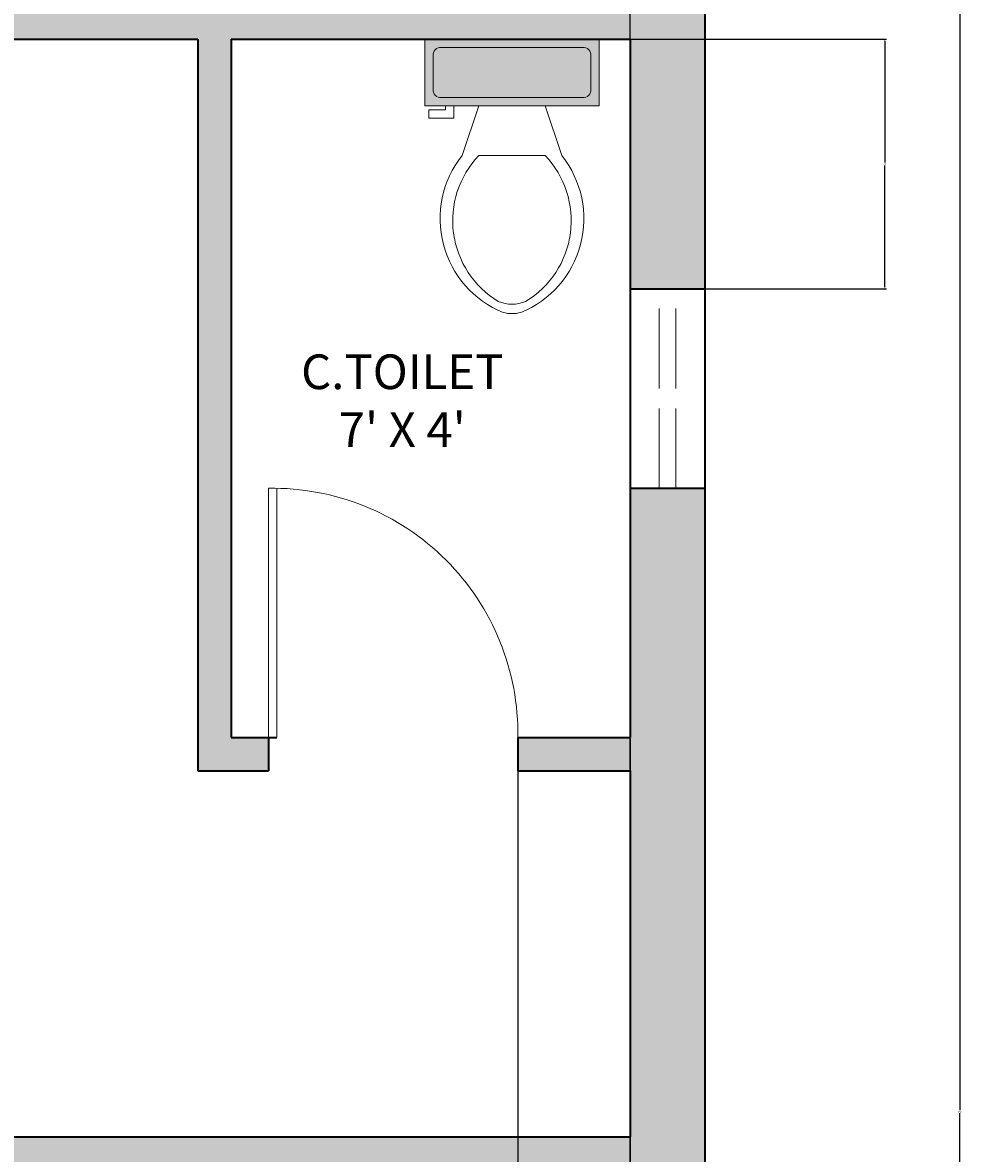
# Model space of a CAD drawing. Units: inches. Extents: x 1567 to 1964, y 1813 to 2447.
# Tile 23 of 28: x 1851 to 1964, y 2125 to 2261. Entities that reach past the tile are written whole.
import ezdxf

# ---------------------------------------------------------------- set-up
doc = ezdxf.new("R2010")
doc.units = ezdxf.units.IN
doc.linetypes.add('ACAD_ISO02W100', pattern=[15, 12, -3])
for name, color, linetype, lineweight in [('A-ANNO-DIMS', 2, 'Continuous', 18), ('A-AREA-IDEN', 7, 'Continuous', 18), ('A-DOOR', 4, 'Continuous', 18), ('A-FLOR-FIXT', 8, 'Continuous', 20), ('A-GLAZ-OVHD', 4, 'ACAD_ISO02W100', 18), ('A-WALL', 7, 'Continuous', 35)]:
    doc.layers.add(name, color=color, linetype=linetype, lineweight=lineweight)
doc.layers.add('A-FURN-PATT', color=252, linetype='Continuous', lineweight=13, true_color=0x939598)
doc.layers.add('A-WALL-PATT', color=251, linetype='Continuous', lineweight=13, true_color=0x636466)
doc.styles.get("Standard").update_dxf_attribs({"font": 'arial.ttf'})
doc.dimstyles.get("Standard").update_dxf_attribs({"dimtxt": 0.18, "dimasz": 0.18, "dimexe": 0.18, "dimexo": 0.0625, "dimgap": 0.09, "dimtad": 0, "dimtih": 1, "dimtoh": 1, "dimdec": 4, "dimzin": 0, "dimdsep": 46, "dimtxsty": 'Standard', "dimcen": 0.09, "dimadec": 0, "dimazin": 0, "dimtfac": 1, "dimtdec": 4, "dimtofl": 0, "dimtmove": 0, "dimatfit": 3, "dimfxl": 1, "dimtolj": 1, "dimtzin": 0, "dimarcsym": 0})

# ---------------------------------------------------------------- blocks, each defined once
blk = doc.blocks.new('Toilet - top')
for p, q in [((9.5, -6), (9.5, -2)), ((-8, -8.5), (-8, -8)), ((-7, -8), (-7, -9.5)), ((-4, -8), (-6, -14)), ((4, -8), (6, -14)), ((-10, -8.5), (-8, -8.5)), ((-10, -9.5), (-10, -8.5)), ((-7, -9.5), (-10, -9.5)), ((4, -14), (-4, -14))]:
    blk.add_line(p, q)
blk.add_lwpolyline([(10.5, -8), (10.5, 0), (-10.5, 0), (-10.5, -8)], close=True)
for points in [[(8.5, -1), (-8.5, -1)], [(-9.5, -2), (-9.5, -6)], [(-8.5, -7), (8.5, -7)]]:
    blk.add_lwpolyline(points)
for centre, radius, start, end in [((-8.62, -1.88), 0.884, 81.8699, 188.1301), ((8.62, -1.88), 0.884, 351.8699, 98.1301), ((-8.62, -6.12), 0.884, 171.8699, 278.1301), ((8.62, -6.12), 0.884, 261.8699, 8.1301), ((3.52, -21.58), 12.17, 141.4691, 247.9714), ((4.2, -21.82), 11.33, 136.3677, 238.9468), ((-3.52, -21.58), 12.17, 292.0284, 38.5307), ((-4.2, -21.82), 11.33, 301.053, 43.6321), ((0, -27.88), 4, 245.7318, 294.2682), ((0, -29), 4, 254.8605, 285.1395)]:
    blk.add_arc(centre, radius, start, end)
blk = doc.blocks.new('DOOR-SWING-30IN')
for p, q in [((0, 0), (0, 30)), ((1, 0), (1, 30))]:
    blk.add_line(p, q)
blk.add_arc((0.5, 0.5), 29.5, 359.029, 90.971)
blk = doc.blocks.new('WINDOW-24IN-HIGH')
at = {"ltscale": 0.8}
for p, q in [((0, 2), (24, 2)), ((0, 0), (24, 0))]:
    blk.add_line(p, q, dxfattribs=at)
blk = doc.blocks.new('*D40')
at = {"layer": 'A-ANNO-DIMS', "color": 0, "lineweight": -2, "transparency": 16777216}
for p, q in [((1933.49, 2416.29), (1964.26, 2416.29)), ((1964.08, 2416.11), (1964.08, 2130.47)), ((1964.08, 1844.47), (1964.08, 2130.11)), ((1933.49, 1844.29), (1964.26, 1844.29))]:
    blk.add_line(p, q, dxfattribs=at)
at = {"layer": 'A-ANNO-DIMS', "color": 0, "transparency": 16777216}
for points in [[(1964.05, 2416.11), (1964.11, 2416.11), (1964.08, 2416.29)], [(1964.05, 1844.47), (1964.11, 1844.47), (1964.08, 1844.29)]]:
    blk.add_solid(points, dxfattribs=at)
at = {"layer": 'Defpoints', "color": 0, "transparency": 16777216}
for p in [(1933.43, 2416.29), (1964.08, 2416.29), (1933.43, 1844.29)]:
    blk.add_point(p, dxfattribs=at)
at = {"layer": 'A-ANNO-DIMS', "color": 0, "transparency": 16777216, "insert": (1964.08, 2130.29), "char_height": 0.18, "attachment_point": 5}
blk.add_mtext('\\A1;572', dxfattribs=at)
blk = doc.blocks.new('*D51')
at = {"layer": 'A-ANNO-DIMS', "color": 0, "lineweight": -2, "transparency": 16777216}
for p, q in [((1924.49, 2259.29), (1955.26, 2259.29)), ((1955.08, 2259.11), (1955.08, 2244.47)), ((1955.08, 2229.47), (1955.08, 2244.11)), ((1924.49, 2229.29), (1955.26, 2229.29))]:
    blk.add_line(p, q, dxfattribs=at)
at = {"layer": 'A-ANNO-DIMS', "color": 0, "transparency": 16777216}
for points in [[(1955.05, 2259.11), (1955.11, 2259.11), (1955.08, 2259.29)], [(1955.05, 2229.47), (1955.11, 2229.47), (1955.08, 2229.29)]]:
    blk.add_solid(points, dxfattribs=at)
at = {"layer": 'Defpoints', "color": 0, "transparency": 16777216}
for p in [(1924.43, 2259.29), (1924.43, 2229.29), (1955.08, 2229.29)]:
    blk.add_point(p, dxfattribs=at)
at = {"layer": 'A-ANNO-DIMS', "color": 0, "transparency": 16777216, "insert": (1955.08, 2244.29), "char_height": 0.18, "attachment_point": 5}
blk.add_mtext('\\A1;30', dxfattribs=at)
blk = doc.blocks.new('*D71')
at = {"layer": 'A-ANNO-DIMS', "color": 0, "lineweight": -2, "transparency": 16777216}
for p, q in [((1799.43, 1910.75), (1799.43, 2447.12)), ((1799.61, 2446.94), (1861.65, 2446.94)), ((1924.25, 2446.94), (1862.21, 2446.94)), ((1924.43, 1910.75), (1924.43, 2447.12))]:
    blk.add_line(p, q, dxfattribs=at)
at = {"layer": 'A-ANNO-DIMS', "color": 0, "transparency": 16777216}
for points in [[(1799.61, 2446.97), (1799.61, 2446.91), (1799.43, 2446.94)], [(1924.25, 2446.97), (1924.25, 2446.91), (1924.43, 2446.94)]]:
    blk.add_solid(points, dxfattribs=at)
at = {"layer": 'Defpoints', "color": 0, "transparency": 16777216}
for p in [(1924.43, 2446.94), (1799.43, 1910.69), (1924.43, 1910.69)]:
    blk.add_point(p, dxfattribs=at)
at = {"layer": 'A-ANNO-DIMS', "color": 0, "transparency": 16777216, "insert": (1861.93, 2446.94), "char_height": 0.18, "attachment_point": 5}
blk.add_mtext('\\A1;125', dxfattribs=at)
blk = doc.blocks.new('*D72')
at = {"layer": 'A-ANNO-DIMS', "color": 0, "lineweight": -2, "transparency": 16777216}
for p, q in [((1910.93, 2175.23), (1910.93, 1813.46)), ((1924.43, 2175.23), (1924.43, 1813.46)), ((1911.11, 1813.64), (1917.36, 1813.64)), ((1924.25, 1813.64), (1918, 1813.64))]:
    blk.add_line(p, q, dxfattribs=at)
at = {"layer": 'A-ANNO-DIMS', "color": 0, "transparency": 16777216}
for points in [[(1911.11, 1813.67), (1911.11, 1813.61), (1910.93, 1813.64)], [(1924.25, 1813.67), (1924.25, 1813.61), (1924.43, 1813.64)]]:
    blk.add_solid(points, dxfattribs=at)
at = {"layer": 'Defpoints', "color": 0, "transparency": 16777216}
for p in [(1910.93, 2175.29), (1924.43, 2175.29), (1924.43, 1813.64)]:
    blk.add_point(p, dxfattribs=at)
at = {"layer": 'A-ANNO-DIMS', "color": 0, "transparency": 16777216, "insert": (1917.68, 1813.64), "char_height": 0.18, "attachment_point": 5}
blk.add_mtext('\\A1;13.5', dxfattribs=at)

msp = doc.modelspace()

# ---------------------------------------------------------------- hatches: boundary and pattern name
at = {"layer": 'A-FURN-PATT'}
h = msp.add_hatch(color=256, dxfattribs=at)
h.dxf.hatch_style = 1
h.paths.add_polyline_path([(1621.2532, 2242.0229), (1643.7811, 2241.7239), (1643.8607, 2247.7234), (1617.863, 2248.0685, 0.19047621), (1616.7481, 2164.0759), (1642.7458, 2163.7308), (1642.8254, 2169.7302), (1620.2975, 2170.0293, -0.15194781)])
h.paths.add_polyline_path([(1673.5306, 2249.6607), (1653.8509, 2249.6607), (1653.8509, 2248.5031, 0.11764706), (1673.5306, 2248.5031)])
h.paths.add_polyline_path([(1706.0889, 2249.6607), (1686.4092, 2249.6607), (1686.4092, 2248.5031, 0.11764706), (1706.0889, 2248.5031)])
h.paths.add_polyline_path([(1782.4511, 2227.4197), (1766.4511, 2227.4197), (1766.2949, 2226.4197), (1782.6074, 2226.4197)])
h.paths.add_polyline_path([(1810.4511, 2227.4197), (1794.4511, 2227.4197), (1794.2949, 2226.4197), (1810.6074, 2226.4197)])
h.paths.add_polyline_path([(1743.9511, 2208.076), (1742.9511, 2207.9197), (1742.9511, 2191.9197), (1743.9511, 2191.7635)])
h.paths.add_polyline_path([(1782.6074, 2173.4197), (1766.2949, 2173.4197), (1766.4511, 2172.4197), (1782.4511, 2172.4197)])
h.paths.add_polyline_path([(1810.6074, 2173.4197), (1794.2949, 2173.4197), (1794.4511, 2172.4197), (1810.4511, 2172.4197)])
h.paths.add_polyline_path([(1861.053, 2006.5071), (1845.8531, 2006.5071), (1861.053, 1991.3071)])
h.paths.add_polyline_path([(1905.853, 1993.7071), (1861.053, 1993.7071), (1861.053, 1991.3071), (1905.853, 1991.3071)])
h.paths.add_polyline_path([(1919.7245, 2257.29, 0.50000012), (1918.7245, 2258.29), (1901.7245, 2258.29, 0.50000012), (1900.7245, 2257.29), (1900.7245, 2253.29, 0.50000012), (1901.7245, 2252.29), (1918.7245, 2252.29, 0.50000012), (1919.7245, 2253.29)])
h.paths.add_polyline_path([(1875.9094, 2391.0204), (1875.9094, 2375.8204), (1891.1093, 2375.8204)], flags=17)
h.paths.add_polyline_path([(1891.1093, 2405.4204), (1831.1094, 2405.4204), (1831.1094, 2391.0204), (1839.1093, 2391.0204), (1839.1093, 2404.2204), (1859.9093, 2404.2204), (1859.9093, 2391.0204), (1862.3093, 2391.0204), (1862.3093, 2404.2204), (1883.1093, 2404.2204), (1883.1093, 2389.0204), (1877.9094, 2389.0204), (1891.1093, 2375.8204)])
h.paths.add_polyline_path([(1682.1402, 2390.0316), (1682.1402, 2374.8316), (1697.3402, 2374.8316)], flags=17)
h.paths.add_polyline_path([(1697.3402, 2404.4316), (1637.3402, 2404.4316), (1637.3402, 2390.0316), (1645.3402, 2390.0316), (1645.3402, 2403.2316), (1666.1402, 2403.2316), (1666.1402, 2390.0316), (1668.5402, 2390.0316), (1668.5402, 2403.2316), (1689.3402, 2403.2316), (1689.3402, 2388.0316), (1684.1402, 2388.0316), (1697.3402, 2374.8316)])
h = msp.add_hatch(color=256, dxfattribs=at)
h.dxf.hatch_style = 1
h.paths.add_polyline_path([(1642.2233, 2241.7446), (1623.1648, 2241.9976), (1622.8462, 2217.9997), (1641.9047, 2217.7467)])
h.paths.add_polyline_path([(1641.9047, 2217.7467), (1622.8462, 2217.9997), (1622.5277, 2194.0018), (1641.5862, 2193.7488)])
h.paths.add_polyline_path([(1641.5862, 2193.7488), (1622.5277, 2194.0018), (1622.2091, 2170.0039), (1641.2677, 2169.7509)])
h.paths.add_polyline_path([(1671.2154, 2243.8726, -0.23606798), (1673.5306, 2245.0302), (1673.5306, 2246.1879), (1653.8509, 2246.1879), (1653.8509, 2245.0302, -0.23606798), (1656.1662, 2243.8726), (1656.1662, 2233.4539, -0.23606798), (1653.8509, 2232.2963), (1653.8509, 2231.1387, 0.11764706), (1673.5306, 2231.1387), (1673.5306, 2232.2963, -0.23606798), (1671.2154, 2233.4539)])
h.paths.add_polyline_path([(1703.7736, 2243.8726, -0.23606798), (1706.0889, 2245.0302), (1706.0889, 2246.1879), (1686.4092, 2246.1879), (1686.4092, 2245.0302, -0.23606798), (1688.7245, 2243.8726), (1688.7245, 2233.4539, -0.23606798), (1686.4092, 2232.2963), (1686.4092, 2231.1387, 0.11764706), (1706.0889, 2231.1387), (1706.0889, 2232.2963, -0.23606798), (1703.7736, 2233.4539)])
h.paths.add_polyline_path([(1782.6855, 2225.9197), (1766.2168, 2225.9197), (1764.9668, 2217.9197), (1783.9356, 2217.9197)])
h.paths.add_polyline_path([(1810.6855, 2225.9197), (1794.2168, 2225.9197), (1792.9668, 2217.9197), (1811.9356, 2217.9197)])
h.paths.add_polyline_path([(1752.4511, 2209.4041), (1744.4511, 2208.1541), (1744.4511, 2191.6853), (1752.4511, 2190.4354)])
h.paths.add_polyline_path([(1783.9356, 2181.9197), (1764.9668, 2181.9197), (1766.2168, 2173.9197), (1782.6855, 2173.9197)])
h.paths.add_polyline_path([(1811.9356, 2181.9197), (1792.9668, 2181.9197), (1794.2168, 2173.9197), (1810.6855, 2173.9197)])
h.paths.add_polyline_path([(1832.4511, 2208.1541), (1824.4511, 2209.4041), (1824.4511, 2190.4354), (1832.4511, 2191.6853)])
h.paths.add_polyline_path([(1824.4511, 2194.4197), (1823.8775, 2194.266), (1823.2838, 2194.1743), (1822.6735, 2194.1363), (1822.0501, 2194.1437), (1821.4169, 2194.1882), (1820.7773, 2194.2615), (1820.1348, 2194.3554), (1819.4928, 2194.4614), (1818.8527, 2194.5726), (1818.2083, 2194.6873), (1817.5511, 2194.8049), (1816.873, 2194.9249), (1816.1656, 2195.0469), (1815.4205, 2195.1704), (1814.6296, 2195.2948), (1813.7845, 2195.4197), (1812.88, 2195.5442), (1811.9238, 2195.6658), (1810.9265, 2195.7815), (1809.899, 2195.8885), (1808.852, 2195.9837), (1807.7962, 2196.0643), (1806.7423, 2196.1273), (1805.7011, 2196.1697), (1804.6806, 2196.1896), (1803.6777, 2196.188), (1802.6865, 2196.1668), (1801.7011, 2196.1281), (1800.7158, 2196.0737), (1799.7245, 2196.0057), (1798.7216, 2195.9259), (1797.7011, 2195.8364), (1796.6564, 2195.7387), (1795.5781, 2195.6333), (1794.4557, 2195.52), (1793.2792, 2195.3989), (1792.0383, 2195.27), (1790.7226, 2195.1333), (1789.3219, 2194.9887), (1787.8261, 2194.8364), (1786.1882, 2194.6764), (1784.2148, 2194.5096), (1781.6759, 2194.3369), (1778.3417, 2194.1593), (1773.9821, 2193.9778), (1768.3671, 2193.7934), (1761.2668, 2193.6071), (1752.4511, 2193.4197), (1752.4511, 2189.9197), (1762.0489, 2190.1067), (1769.9836, 2190.2908), (1776.4672, 2190.469), (1781.7115, 2190.6385), (1785.9285, 2190.7962), (1789.33, 2190.9393), (1792.128, 2191.0648), (1794.5344, 2191.1697), (1796.7278, 2191.2521), (1798.7532, 2191.313), (1800.6223, 2191.3543), (1802.3469, 2191.3781), (1803.9387, 2191.3862), (1805.4094, 2191.3807), (1806.7708, 2191.3634), (1808.0345, 2191.3364), (1809.2127, 2191.3013), (1810.3196, 2191.2589), (1811.3699, 2191.2097), (1812.3782, 2191.1541), (1813.3592, 2191.0927), (1814.3274, 2191.0259), (1815.2976, 2190.9542), (1816.2845, 2190.8781), (1817.2985, 2190.7986), (1818.3339, 2190.7186), (1819.3811, 2190.6415), (1820.4303, 2190.5708), (1821.4716, 2190.5098), (1822.4954, 2190.4621), (1823.4918, 2190.4309), (1824.3581, 2190.4208), (1824.4511, 2190.4354)])
h.paths.add_polyline_path([(1874.6531, 1991.3071), (1861.053, 1991.3071), (1859.053, 1993.3071), (1853.8531, 1993.3071), (1853.8531, 1978.1071), (1874.6531, 1978.1071)], flags=17)
h.paths.add_polyline_path([(1897.8531, 1991.3071), (1877.0531, 1991.3071), (1877.0531, 1978.1071), (1897.8531, 1978.1071)], flags=17)
h.paths.add_polyline_path([(1853.8531, 1993.3071), (1859.053, 1993.3071), (1845.8531, 2006.5071), (1845.8531, 1976.9071), (1905.853, 1976.9071), (1905.853, 1991.3071), (1897.8531, 1991.3071), (1897.8531, 1978.1071), (1877.0531, 1978.1071), (1877.0531, 1991.3071), (1874.6531, 1991.3071), (1874.6531, 1978.1071), (1853.8531, 1978.1071)])
h.paths.add_polyline_path([(1920.7245, 2259.29), (1899.7245, 2259.29), (1899.7245, 2251.29), (1920.7245, 2251.29)])
h.paths.add_polyline_path([(1918.7245, 2252.29, 0.50000012), (1919.7245, 2253.29), (1919.7245, 2257.29, 0.50000012), (1918.7245, 2258.29), (1901.7245, 2258.29, 0.50000012), (1900.7245, 2257.29), (1900.7245, 2253.29, 0.50000012), (1901.7245, 2252.29)], flags=16)
h.paths.add_polyline_path([(1843.2327, 2065.967), (1919.26, 2065.967), (1919.26, 2095.8187), (1843.2327, 2095.8187)], flags=9)
at = {"layer": 'A-WALL-PATT'}
h = msp.add_hatch(color=256, dxfattribs=at)
h.dxf.hatch_style = 1
h.paths.add_polyline_path([(1606.4295, 2407.29), (1654.4295, 2407.29), (1654.4295, 2416.29), (1597.4295, 2416.29), (1597.4295, 2217.29), (1606.4295, 2217.29), (1606.4295, 2259.29), (1738.4295, 2259.29), (1738.4295, 2247.29), (1742.4295, 2247.29), (1742.4295, 2259.29), (1742.4295, 2272.29), (1738.4295, 2272.29), (1738.4295, 2263.29), (1606.4295, 2263.29)])
h.paths.add_polyline_path([(1753.4295, 2416.29), (1690.4295, 2416.29), (1690.4295, 2407.29), (1738.4295, 2407.29), (1738.4295, 2308.29), (1742.4295, 2308.29), (1742.4295, 2331.29), (1746.9295, 2331.29), (1746.9295, 2335.29), (1742.4295, 2335.29), (1742.4295, 2407.29), (1753.4295, 2407.29)])
h.paths.add_polyline_path([(1840.4295, 2416.29), (1777.4295, 2416.29), (1777.4295, 2407.29), (1788.4295, 2407.29), (1788.4295, 2335.29), (1776.9295, 2335.29), (1776.9295, 2331.29), (1788.4295, 2331.29), (1788.4295, 2308.29), (1792.4295, 2308.29), (1792.4295, 2407.29), (1840.4295, 2407.29)])
h.paths.add_polyline_path([(1933.4295, 2416.29), (1876.4295, 2416.29), (1876.4295, 2407.29), (1924.4295, 2407.29), (1924.4295, 2263.29), (1792.4295, 2263.29), (1792.4295, 2272.29), (1788.4295, 2272.29), (1788.4295, 2259.29), (1872.4295, 2259.29), (1872.4295, 2171.29), (1880.9295, 2171.29), (1880.9295, 2175.29), (1876.4295, 2175.29), (1876.4295, 2259.29), (1924.4295, 2259.29), (1924.4295, 2229.29), (1933.4295, 2229.29)])
h.paths.add_polyline_path([(1933.4295, 2205.29), (1924.4295, 2205.29), (1924.4295, 2175.29), (1910.9295, 2175.29), (1910.9295, 2171.29), (1924.4295, 2171.29), (1924.4295, 2127.29), (1844.4295, 2127.29), (1844.4295, 2123.29), (1924.4295, 2123.29), (1924.4295, 2063.29), (1933.4295, 2063.29)])
h.paths.add_polyline_path([(1799.4295, 2123.29), (1808.4295, 2123.29), (1808.4295, 2127.29), (1781.4295, 2127.29), (1781.4295, 2123.29), (1795.4295, 2123.29), (1795.4295, 1964.29), (1711.4295, 1964.29), (1711.4295, 2123.29), (1751.4295, 2123.29), (1751.4295, 2127.29), (1742.4295, 2127.29), (1742.4295, 2139.29), (1738.4295, 2139.29), (1738.4295, 2127.29), (1678.4295, 2127.29), (1678.4295, 2123.29), (1702.4295, 2123.29), (1702.4295, 1913.29), (1678.4295, 1913.29), (1678.4295, 1904.29), (1711.4295, 1904.29), (1711.4295, 1960.29), (1795.4295, 1960.29), (1795.4295, 1906.69), (1929.4295, 1906.69), (1929.4295, 1848.29), (1601.4295, 1848.29), (1601.4295, 1904.29), (1630.4295, 1904.29), (1630.4295, 1913.29), (1606.4295, 1913.29), (1606.4295, 2123.29), (1630.4295, 2123.29), (1630.4295, 2127.29), (1606.4295, 2127.29), (1606.4295, 2169.29), (1597.4295, 2169.29), (1597.4295, 1844.29), (1933.4295, 1844.29), (1933.4295, 2027.29), (1924.4295, 2027.29), (1924.4295, 1967.29), (1833.9295, 1967.29), (1833.9295, 1963.29), (1924.4295, 1963.29), (1924.4295, 1910.69), (1799.4295, 1910.69), (1799.4295, 1963.29), (1803.9295, 1963.29), (1803.9295, 1967.29), (1799.4295, 1967.29)])

# ---------------------------------------------------------------- linework, layer by layer
at = {"layer": 'A-WALL'}
for p, q in [((1933.4295, 2416.29), (1933.4295, 1844.29)), ((1788.4295, 2259.29), (1872.4295, 2259.29)), ((1872.4295, 2259.29), (1872.4295, 2171.29)), ((1876.4295, 2259.29), (1876.4295, 2175.29)), ((1876.4295, 2259.29), (1924.4295, 2259.29)), ((1924.4295, 2259.29), (1924.4295, 2175.29)), ((1924.4295, 2229.29), (1933.4295, 2229.29)), ((1924.4295, 2205.29), (1933.4295, 2205.29)), ((1876.4295, 2175.29), (1881.9295, 2175.29)), ((1880.9295, 2175.29), (1880.9295, 2171.29)), ((1910.9295, 2175.29), (1910.9295, 2171.29)), ((1910.9295, 2175.29), (1924.4295, 2175.29)), ((1872.4295, 2171.29), (1880.9295, 2171.29)), ((1910.9295, 2171.29), (1924.4295, 2171.29)), ((1924.4295, 2171.29), (1924.4295, 2127.29)), ((1844.4295, 2127.29), (1924.4295, 2127.29))]:
    msp.add_line(p, q, dxfattribs=at)

# ---------------------------------------------------------------- block references
at = {"layer": 'A-DOOR'}
msp.add_blockref('DOOR-SWING-30IN', (1880.93, 2175.29), dxfattribs=at)
at = {"layer": 'A-FLOR-FIXT'}
msp.add_blockref('Toilet - top', (1910.2245, 2259.29), dxfattribs=at)
at = {"layer": 'A-GLAZ-OVHD', "rotation": 90.00000000000003}
msp.add_blockref('WINDOW-24IN-HIGH', (1929.9295, 2205.2905), dxfattribs=at)

# ---------------------------------------------------------------- texts
at = {"layer": 'A-AREA-IDEN', "insert": (1875.7252, 2221.3806), "char_height": 4.16967, "attachment_point": 1}
msp.add_mtext_dynamic_manual_height_columns("\\pxqc;C.TOILET\\P7' X 4'", width=42.610804, gutter_width=6.5151, heights=[0], dxfattribs=at)

# ---------------------------------------------------------------- dimensions: what is measured, and where the dimension line sits
at = {"layer": 'A-ANNO-DIMS'}
for base, p1, p2, override, picture, middle in [((1924.4295, 2446.94), (1799.4295, 1910.69), (1924.4295, 1910.69), {"dimdec": 0, "dimlfac": 1, "dimrnd": 0, "dimzin": 0, "dimdsep": 46, "dimlunit": 2}, '*D71', (1861.9295, 2446.94)), ((1924.4295, 1813.64), (1910.9295, 2175.29), (1924.4295, 2175.29), {"dimdec": 1, "dimlfac": 1, "dimrnd": 0, "dimzin": 0, "dimdsep": 46, "dimlunit": 2}, '*D72', (1917.6795, 1813.64))]:
    dim = msp.add_linear_dim(base=base, p1=p1, p2=p2, dimstyle='Standard', override=override, dxfattribs=at)
    dim.commit()
    dim.dimension.update_dxf_attribs({"geometry": picture, "text_midpoint": middle})
for base, p1, p2, angle, picture, middle in [((1964.0795, 2416.29), (1933.4295, 1844.29), (1933.4295, 2416.29), 90, '*D40', (1964.0795, 2130.29)), ((1955.0795, 2229.29), (1924.4295, 2259.29), (1924.4295, 2229.29), 270, '*D51', (1955.0795, 2244.29))]:
    dim = msp.add_linear_dim(base=base, p1=p1, p2=p2, angle=angle, dimstyle='Standard', override={"dimdec": 0, "dimlfac": 1, "dimrnd": 0, "dimzin": 0, "dimdsep": 46, "dimlunit": 2}, dxfattribs=at)
    dim.commit()
    dim.dimension.update_dxf_attribs({"geometry": picture, "text_midpoint": middle})

doc.saveas('drawing.dxf')
